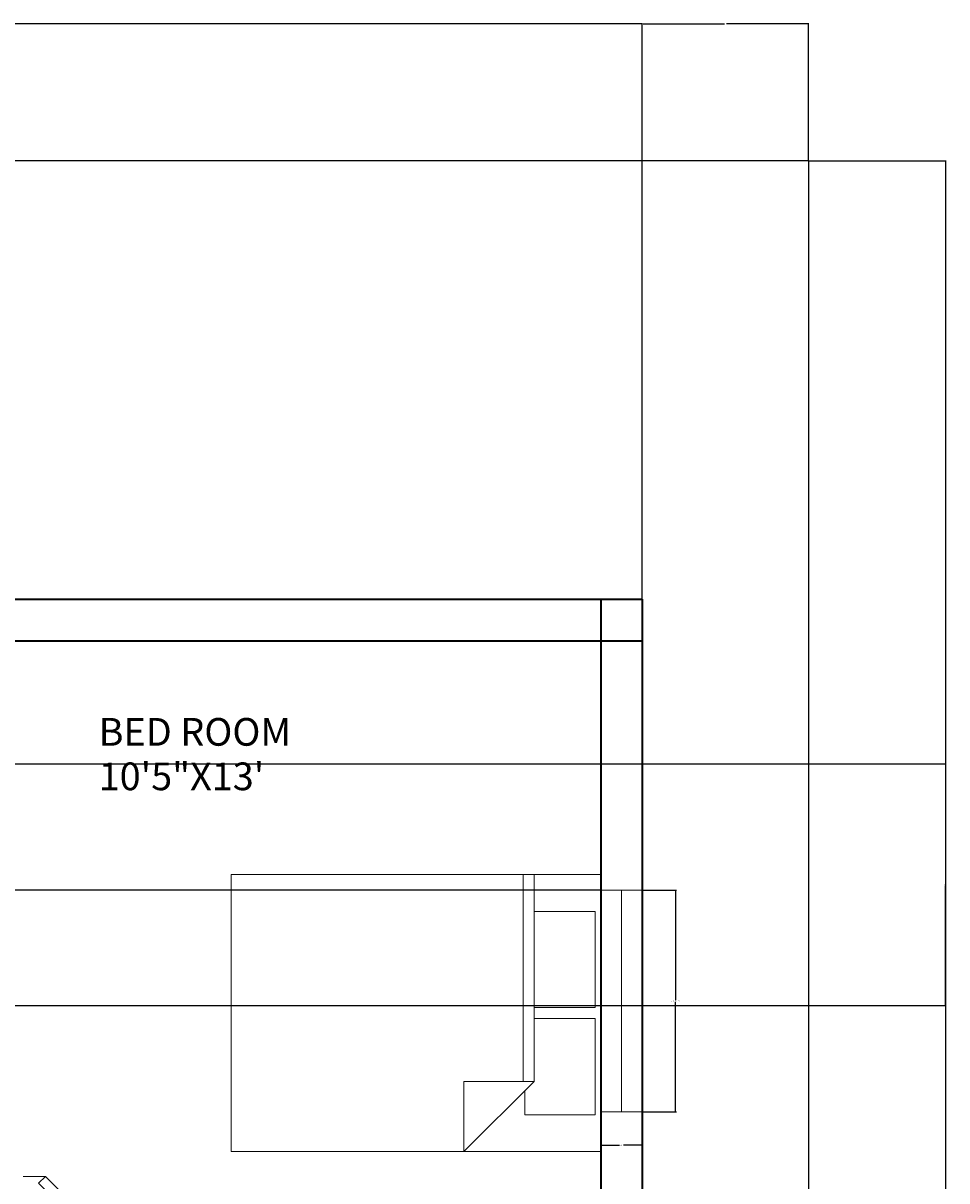
# Model space of a CAD drawing. Units: inches. Extents: x 450 to 1026, y 542 to 1190.
# Tile 11 of 11: x 826 to 1026, y 939 to 1190. Entities that reach past the tile are written whole.
import ezdxf

# ---------------------------------------------------------------- set-up
doc = ezdxf.new("R2010")
doc.units = ezdxf.units.IN
doc.header["$MEASUREMENT"] = 0
for name, color, linetype, lineweight in [('A-ANNO-DIMS', 2, 'Continuous', 18), ('A-AREA-IDEN', 7, 'Continuous', 18), ('A-DOOR', 4, 'Continuous', 18), ('A-FURN', 8, 'Continuous', 18), ('A-GLAZ', 4, 'Continuous', 18), ('A-WALL', 7, 'Continuous', 35), ('C-PROP', 7, 'Continuous', 25)]:
    doc.layers.add(name, color=color, linetype=linetype, lineweight=lineweight)
doc.styles.get("Standard").update_dxf_attribs({"font": 'arial.ttf'})
doc.dimstyles.get("Standard").update_dxf_attribs({"dimtxt": 0.18, "dimasz": 0.18, "dimexe": 0.18, "dimexo": 0.0625, "dimgap": 0.09, "dimtad": 0, "dimtih": 1, "dimtoh": 1, "dimdec": 4, "dimzin": 0, "dimdsep": 46, "dimtxsty": 'Standard', "dimcen": 0.09, "dimadec": 0, "dimazin": 0, "dimtfac": 1, "dimtdec": 4, "dimtofl": 0, "dimtmove": 0, "dimatfit": 3, "dimfxl": 1, "dimtolj": 1, "dimtzin": 0, "dimarcsym": 0})

# ---------------------------------------------------------------- blocks, each defined once
blk = doc.blocks.new('*U4')
for p, q in [((0, 0), (0, -100)), ((750, 0), (750, -100))]:
    blk.add_line(p, q)
blk.add_lwpolyline([(0, 0), (530.3, 530.3), (561.3, 499.4), (30.9, -30.9)], close=True)
blk.add_arc((0, 0), 750, 0, 45)
blk = doc.blocks.new('*U3')
for p, q in [((0, 100), (0, 0)), ((900, 100), (900, 0)), ((0, 50), (900, 50))]:
    blk.add_line(p, q)
blk = doc.blocks.new('Bed - Queen')
for p, q in [((0, -80.00003), (0, 0)), ((0, 0), (59.99999, 0)), ((59.99999, 0), (59.99999, -80.00003)), ((7.99999, -1.2), (28.79998, -1.2)), ((7.99999, -14.4), (7.99999, -1.2)), ((28.79998, -1.2), (28.79998, -14.4)), ((31.19999, -1.2), (51.99999, -1.2)), ((31.19999, -14.4), (31.19999, -1.2)), ((51.99999, -1.2), (51.99999, -16.4)), ((0, -14.4), (44.8, -14.4)), ((59.99999, -29.6), (44.8, -14.4)), ((44.8, -14.4), (44.8, -29.6)), ((44.8, -16.8), (0, -16.8)), ((51.99999, -16.4), (46.79936, -16.4)), ((44.8, -29.6), (59.99999, -29.6)), ((59.99999, -80.00003), (0, -80.00003))]:
    blk.add_line(p, q)
blk = doc.blocks.new('WIN-FRAME-48IN')
for p, q in [((9, 48), (0, 48)), ((9, 0), (9, 48)), ((0, 0), (9, 0))]:
    blk.add_line(p, q)
blk = doc.blocks.new('*D35')
at = {"layer": 'A-ANNO-DIMS', "color": 0, "lineweight": -2, "transparency": 16777216}
for p, q in [((959.71, 1001.94), (967.03, 1001.94)), ((966.85, 1001.76), (966.85, 978.13)), ((966.85, 954.12), (966.85, 977.76)), ((959.71, 953.94), (967.03, 953.94))]:
    blk.add_line(p, q, dxfattribs=at)
at = {"layer": 'A-ANNO-DIMS', "color": 0, "transparency": 16777216}
for points in [[(966.82, 1001.76), (966.88, 1001.76), (966.85, 1001.94)], [(966.82, 954.12), (966.88, 954.12), (966.85, 953.94)]]:
    blk.add_solid(points, dxfattribs=at)
at = {"layer": 'Defpoints', "color": 0, "transparency": 16777216}
for p in [(959.65, 1001.94), (966.85, 1001.94), (959.65, 953.94)]:
    blk.add_point(p, dxfattribs=at)
at = {"layer": 'A-ANNO-DIMS', "color": 0, "transparency": 16777216, "insert": (966.85, 977.94), "char_height": 0.18, "attachment_point": 5}
blk.add_mtext('\\A1;WINDOW 48 TYP.', dxfattribs=at)
blk = doc.blocks.new('*D36')
at = {"layer": 'A-ANNO-DIMS', "color": 0, "lineweight": -2, "transparency": 16777216}
for p, q in [((950.65, 953.88), (950.65, 946.56)), ((959.65, 953.88), (959.65, 946.56)), ((950.83, 946.74), (954.69, 946.74)), ((959.47, 946.74), (955.61, 946.74))]:
    blk.add_line(p, q, dxfattribs=at)
at = {"layer": 'A-ANNO-DIMS', "color": 0, "transparency": 16777216}
for points in [[(950.83, 946.77), (950.83, 946.71), (950.65, 946.74)], [(959.47, 946.77), (959.47, 946.71), (959.65, 946.74)]]:
    blk.add_solid(points, dxfattribs=at)
at = {"layer": 'Defpoints', "color": 0, "transparency": 16777216}
for p in [(950.65, 953.94), (959.65, 953.94), (959.65, 946.74)]:
    blk.add_point(p, dxfattribs=at)
at = {"layer": 'A-ANNO-DIMS', "color": 0, "transparency": 16777216, "insert": (955.15, 946.74), "char_height": 0.18, "attachment_point": 5}
blk.add_mtext('\\A1;9 TYP.', dxfattribs=at)
blk = doc.blocks.new('*D46')
at = {"layer": 'A-ANNO-DIMS', "color": 0, "lineweight": -2, "transparency": 16777216}
for p, q in [((995.71, 1159.94), (1025.43, 1159.94)), ((1025.25, 1159.76), (1025.25, 866.12)), ((1025.25, 572.12), (1025.25, 865.76)), ((995.71, 571.94), (1025.43, 571.94))]:
    blk.add_line(p, q, dxfattribs=at)
at = {"layer": 'A-ANNO-DIMS', "color": 0, "transparency": 16777216}
for points in [[(1025.22, 1159.76), (1025.28, 1159.76), (1025.25, 1159.94)], [(1025.22, 572.12), (1025.28, 572.12), (1025.25, 571.94)]]:
    blk.add_solid(points, dxfattribs=at)
at = {"layer": 'Defpoints', "color": 0, "transparency": 16777216}
for p in [(995.65, 1159.94), (1025.25, 1159.94), (995.65, 571.94)]:
    blk.add_point(p, dxfattribs=at)
at = {"layer": 'A-ANNO-DIMS', "color": 0, "transparency": 16777216, "insert": (1025.25, 865.94), "char_height": 0.18, "attachment_point": 5}
blk.add_mtext('\\A1;588', dxfattribs=at)
blk = doc.blocks.new('*D47')
at = {"layer": 'A-ANNO-DIMS', "color": 0, "lineweight": -2, "transparency": 16777216}
for p, q in [((479.65, 1160.01), (479.65, 1189.72)), ((479.83, 1189.54), (719.36, 1189.54)), ((959.47, 1189.54), (719.94, 1189.54)), ((959.65, 1065.01), (959.65, 1189.72))]:
    blk.add_line(p, q, dxfattribs=at)
at = {"layer": 'A-ANNO-DIMS', "color": 0, "transparency": 16777216}
for points in [[(479.83, 1189.57), (479.83, 1189.51), (479.65, 1189.54)], [(959.47, 1189.57), (959.47, 1189.51), (959.65, 1189.54)]]:
    blk.add_solid(points, dxfattribs=at)
at = {"layer": 'Defpoints', "color": 0, "transparency": 16777216}
for p in [(959.65, 1189.54), (479.65, 1159.94), (959.65, 1064.94)]:
    blk.add_point(p, dxfattribs=at)
at = {"layer": 'A-ANNO-DIMS', "color": 0, "transparency": 16777216, "insert": (719.65, 1189.54), "char_height": 0.18, "attachment_point": 5}
blk.add_mtext('\\A1;480', dxfattribs=at)
blk = doc.blocks.new('*D48')
at = {"layer": 'A-ANNO-DIMS', "color": 0, "lineweight": -2, "transparency": 16777216}
for p, q in [((959.65, 1065.01), (959.65, 1189.72)), ((959.83, 1189.54), (977.43, 1189.54)), ((995.47, 1189.54), (977.87, 1189.54)), ((995.65, 1160.01), (995.65, 1189.72))]:
    blk.add_line(p, q, dxfattribs=at)
at = {"layer": 'A-ANNO-DIMS', "color": 0, "transparency": 16777216}
for points in [[(959.83, 1189.57), (959.83, 1189.51), (959.65, 1189.54)], [(995.47, 1189.57), (995.47, 1189.51), (995.65, 1189.54)]]:
    blk.add_solid(points, dxfattribs=at)
at = {"layer": 'Defpoints', "color": 0, "transparency": 16777216}
for p in [(995.65, 1189.54), (995.65, 1159.94), (959.65, 1064.94)]:
    blk.add_point(p, dxfattribs=at)
at = {"layer": 'A-ANNO-DIMS', "color": 0, "transparency": 16777216, "insert": (977.65, 1189.54), "char_height": 0.18, "attachment_point": 5}
blk.add_mtext('\\A1;36', dxfattribs=at)
blk = doc.blocks.new('*D55')
at = {"layer": 'A-ANNO-DIMS', "color": 0, "lineweight": -2, "transparency": 16777216}
for p, q in [((995.59, 1159.94), (449.87, 1159.94)), ((450.05, 1159.76), (450.05, 1112.62)), ((450.05, 1065.12), (450.05, 1112.26)), ((959.59, 1064.94), (449.87, 1064.94))]:
    blk.add_line(p, q, dxfattribs=at)
at = {"layer": 'A-ANNO-DIMS', "color": 0, "transparency": 16777216}
for points in [[(450.02, 1159.76), (450.08, 1159.76), (450.05, 1159.94)], [(450.02, 1065.12), (450.08, 1065.12), (450.05, 1064.94)]]:
    blk.add_solid(points, dxfattribs=at)
at = {"layer": 'Defpoints', "color": 0, "transparency": 16777216}
for p in [(995.65, 1159.94), (450.05, 1064.94), (959.65, 1064.94)]:
    blk.add_point(p, dxfattribs=at)
at = {"layer": 'A-ANNO-DIMS', "color": 0, "transparency": 16777216, "insert": (450.05, 1112.44), "char_height": 0.18, "attachment_point": 5}
blk.add_mtext('\\A1;95', dxfattribs=at)
blk = doc.blocks.new('*D68')
at = {"layer": 'A-ANNO-DIMS', "color": 0, "lineweight": -2, "transparency": 16777216}
for p, q in [((523.29, 1029.33), (1025.43, 1029.33)), ((1025.25, 1029.15), (1025.25, 1003.32)), ((1025.25, 977.12), (1025.25, 1002.96)), ((523.29, 976.94), (1025.43, 976.94))]:
    blk.add_line(p, q, dxfattribs=at)
at = {"layer": 'A-ANNO-DIMS', "color": 0, "transparency": 16777216}
for points in [[(1025.22, 1029.15), (1025.28, 1029.15), (1025.25, 1029.33)], [(1025.22, 977.12), (1025.28, 977.12), (1025.25, 976.94)]]:
    blk.add_solid(points, dxfattribs=at)
at = {"layer": 'Defpoints', "color": 0, "transparency": 16777216}
for p in [(523.22, 1029.33), (1025.25, 1029.33), (523.22, 976.94)]:
    blk.add_point(p, dxfattribs=at)
at = {"layer": 'A-ANNO-DIMS', "color": 0, "transparency": 16777216, "insert": (1025.25, 1003.14), "char_height": 0.18, "attachment_point": 5}
blk.add_mtext('\\A1;52.39', dxfattribs=at)
blk = doc.blocks.new('*D74')
at = {"layer": 'A-ANNO-DIMS', "color": 0, "lineweight": -2, "transparency": 16777216}
for p, q in [((959.59, 1055.94), (449.87, 1055.94)), ((450.05, 1055.76), (450.05, 1029.12)), ((450.05, 1002.12), (450.05, 1028.76)), ((950.59, 1001.94), (449.87, 1001.94))]:
    blk.add_line(p, q, dxfattribs=at)
at = {"layer": 'A-ANNO-DIMS', "color": 0, "transparency": 16777216}
for points in [[(450.02, 1055.76), (450.08, 1055.76), (450.05, 1055.94)], [(450.02, 1002.12), (450.08, 1002.12), (450.05, 1001.94)]]:
    blk.add_solid(points, dxfattribs=at)
at = {"layer": 'Defpoints', "color": 0, "transparency": 16777216}
for p in [(450.05, 1055.94), (959.65, 1055.94), (950.65, 1001.94)]:
    blk.add_point(p, dxfattribs=at)
at = {"layer": 'A-ANNO-DIMS', "color": 0, "transparency": 16777216, "insert": (450.05, 1028.94), "char_height": 0.18, "attachment_point": 5}
blk.add_mtext('\\A1;54', dxfattribs=at)

msp = doc.modelspace()

# ---------------------------------------------------------------- linework, layer by layer
at = {"layer": 'A-WALL'}
for p, q in [((732.6513, 1064.9426), (959.6513, 1064.9426)), ((950.6513, 1064.9426), (950.6513, 821.9426)), ((959.6513, 1064.9426), (959.6513, 594.9426)), ((732.6513, 1055.9426), (959.6513, 1055.9426))]:
    msp.add_line(p, q, dxfattribs=at)
at = {"layer": 'C-PROP'}
for p, q in [((479.6513, 1159.9426), (995.6513, 1159.9426)), ((995.6513, 1159.9426), (995.6513, 571.9426))]:
    msp.add_line(p, q, dxfattribs=at)

# ---------------------------------------------------------------- block references
at = {"layer": 'A-DOOR', "xscale": 0.048, "yscale": 0.048, "zscale": 0.048, "rotation": 270}
msp.add_blockref('*U4', (830.4513, 939.9426), dxfattribs=at)
at = {"layer": 'A-FURN', "rotation": 270.0000000000108}
msp.add_blockref('Bed - Queen', (950.6513, 1005.3242), dxfattribs=at)
at = {"layer": 'A-GLAZ'}
msp.add_blockref('WIN-FRAME-48IN', (950.651, 953.943), dxfattribs=at)
at = {"layer": 'A-GLAZ', "xscale": 0.0533333333333333, "yscale": 0.0533333333333333, "zscale": 0.0533333333333333, "rotation": 270}
msp.add_blockref('*U3', (952.4847, 1001.9426), dxfattribs=at)

# ---------------------------------------------------------------- texts
at = {"layer": 'A-AREA-IDEN'}
for s, p in [('BED ROOM ', (841.993, 1033.2368)), ('10\'5"X13\'', (841.993, 1023.5983))]:
    msp.add_text(s, height=6, dxfattribs=at).set_placement(p)

# ---------------------------------------------------------------- dimensions: what is measured, and where the dimension line sits
at = {"layer": 'A-ANNO-DIMS'}
for base, p1, p2, picture, middle in [((959.6513, 1189.5426), (479.6513, 1159.9426), (959.6513, 1064.9426), '*D47', (719.6513, 1189.5426)), ((995.6513, 1189.5426), (959.6513, 1064.9426), (995.6513, 1159.9426), '*D48', (977.6513, 1189.5426))]:
    dim = msp.add_linear_dim(base=base, p1=p1, p2=p2, dimstyle='Standard', override={"dimdec": 0, "dimlfac": 1, "dimrnd": 0, "dimzin": 0, "dimdsep": 46, "dimlunit": 2}, dxfattribs=at)
    dim.commit()
    dim.dimension.update_dxf_attribs({"geometry": picture, "text_midpoint": middle})
for base, p1, p2, override, picture, middle in [((450.0513, 1064.9426), (995.6513, 1159.9426), (959.6513, 1064.9426), {"dimdec": 0, "dimlfac": 1, "dimrnd": 0, "dimzin": 0, "dimdsep": 46, "dimlunit": 2}, '*D55', (450.0513, 1112.4426)), ((1025.2513, 1159.9426), (995.6513, 571.9426), (995.6513, 1159.9426), {"dimdec": 0, "dimlfac": 1, "dimrnd": 0, "dimzin": 0, "dimdsep": 46, "dimlunit": 2}, '*D46', (1025.2513, 865.9426)), ((450.0513, 1055.9426), (950.6513, 1001.9426), (959.6513, 1055.9426), {"dimdec": 0, "dimlfac": 1, "dimrnd": 0, "dimzin": 0, "dimdsep": 46, "dimlunit": 2}, '*D74', (450.0513, 1028.9426)), ((1025.2513, 1029.3314), (523.2237, 976.9426), (523.2237, 1029.3314), {"dimdec": 2, "dimlfac": 1, "dimrnd": 0, "dimzin": 0, "dimdsep": 46, "dimlunit": 2}, '*D68', (1025.2513, 1003.137))]:
    dim = msp.add_linear_dim(base=base, p1=p1, p2=p2, angle=90, dimstyle='Standard', override=override, dxfattribs=at)
    dim.commit()
    dim.dimension.update_dxf_attribs({"geometry": picture, "text_midpoint": middle})
dim = msp.add_linear_dim(base=(966.8513, 1001.9426), p1=(959.6513, 953.9426), p2=(959.6513, 1001.9426), angle=90, text='WINDOW <> TYP.', dimstyle='Standard', override={"dimdec": 0, "dimlfac": 1, "dimrnd": 0, "dimzin": 0, "dimdsep": 46, "dimlunit": 2}, dxfattribs=at)
dim.commit()
dim.dimension.update_dxf_attribs({"geometry": '*D35', "text_midpoint": (966.8513, 977.9426)})
dim = msp.add_linear_dim(base=(959.6513, 946.7426), p1=(950.6513, 953.9426), p2=(959.6513, 953.9426), text='<> TYP.', dimstyle='Standard', override={"dimdec": 0, "dimlfac": 1, "dimrnd": 0, "dimzin": 0, "dimdsep": 46, "dimlunit": 2}, dxfattribs=at)
dim.commit()
dim.dimension.update_dxf_attribs({"geometry": '*D36', "text_midpoint": (955.1513, 946.7426)})

doc.saveas('drawing.dxf')
